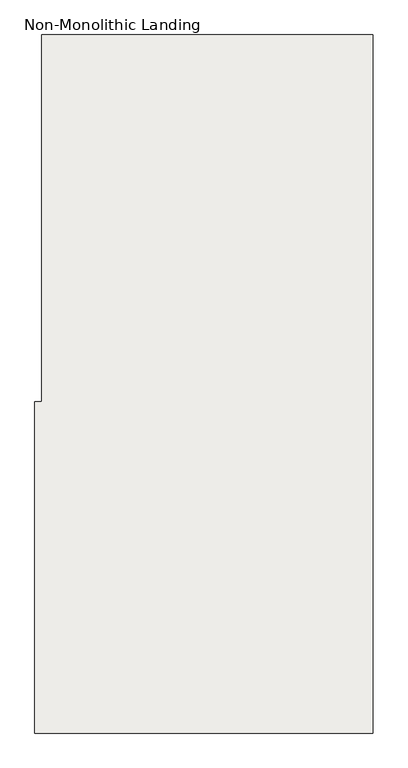
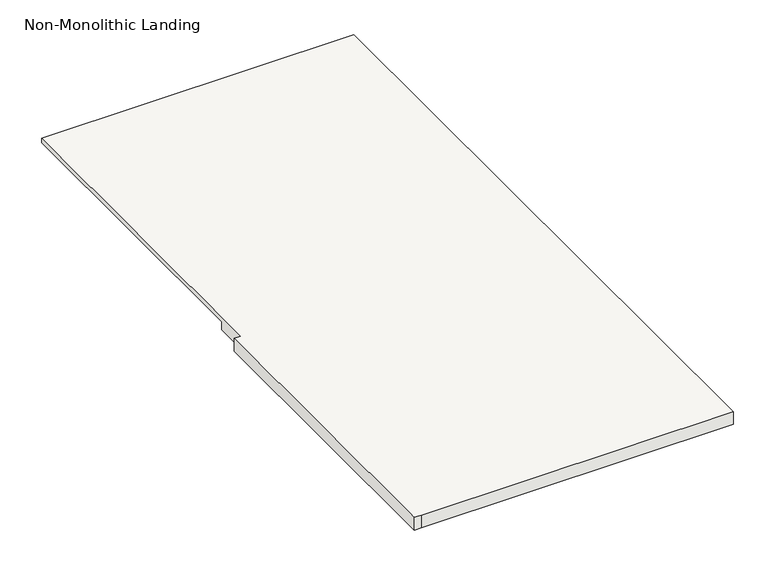
"""IFC4 building model written with IfcOpenShell, lengths in millimetres: slab geometry, Non-Monolithic Landing."""

from ifc_helpers import new_model, si_unit, origin, place, context, project, spatial, faceted_brep, source, transform, mapped, element, save


def non_monolithic_landing_1be43128(model_context):
    return source(origin(), model_context, "Body", "Brep", [
        faceted_brep([(-9863.4532683, 3361.8393562, 1650.723913), (-9838.0532683, 3361.8393562, 1625.323913), (-9838.0532683, 2168.0393562, 1625.323913), (-9863.4532683, 2168.0393562, 1650.723913), (-9863.4532683, 2041.0393562, 1669.773913), (-9888.8532683, 2041.0393562, 1669.773913), (-9888.8532683, 847.2393562, 1669.773913), (-9863.4532683, 847.2393562, 1669.773913), (-8669.6532683, 847.2393562, 1669.773913), (-8669.6532683, 3361.8393562, 1669.773913), (-9863.4532683, 3361.8393562, 1669.773913), (-9838.0532683, 2168.0393562, 1618.973913), (-9838.0532683, 3361.8393562, 1618.973913), (-8669.6532683, 3361.8393562, 1618.973913), (-8669.6532683, 847.2393562, 1618.973913), (-9863.4532683, 847.2393562, 1618.973913), (-9888.8532683, 847.2393562, 1618.973913), (-9888.8532683, 2041.0393562, 1618.973913), (-9863.4532683, 2041.0393562, 1618.973913), (-9863.4532683, 2168.0393562, 1618.973913)], [[[0, 1, 2, 3]], [[4, 5, 6, 7, 8, 9, 10]], [[11, 12, 13, 14, 15, 16, 17, 18, 19]], [[12, 11, 2, 1]], [[11, 19, 3, 2]], [[4, 10, 0, 3, 19, 18]], [[5, 4, 18, 17]], [[6, 5, 17, 16]], [[7, 6, 16, 15]], [[8, 7, 15, 14]], [[9, 8, 14, 13]], [[10, 9, 13, 12, 1, 0]]]),
    ])


if __name__ == "__main__":
    model = new_model("IFC4")
    model_context = context("Model", 3, world=origin())
    ifc_project = project(units=[si_unit("LENGTHUNIT", "METRE", prefix="MILLI")], contexts=[model_context])
    site = spatial("IfcSite", under=ifc_project)
    building = spatial("IfcBuilding", under=site)
    placement = place(None, origin())
    non_monolithic_landing_shape = non_monolithic_landing_1be43128(model_context)
    element("IfcSlab", 1, ObjectType="Non-Monolithic Landing", at=placement, inside=building, context=model_context, shape_type="MappedRepresentation", body=[
        mapped(non_monolithic_landing_shape, transform((0.0, 0.0, 0.0), x_axis=(1.0, 0.0, 0.0), y_axis=(0.0, 1.0, 0.0), z_axis=(0.0, 0.0, 1.0))),
    ])
    save(model, "model.ifc")
